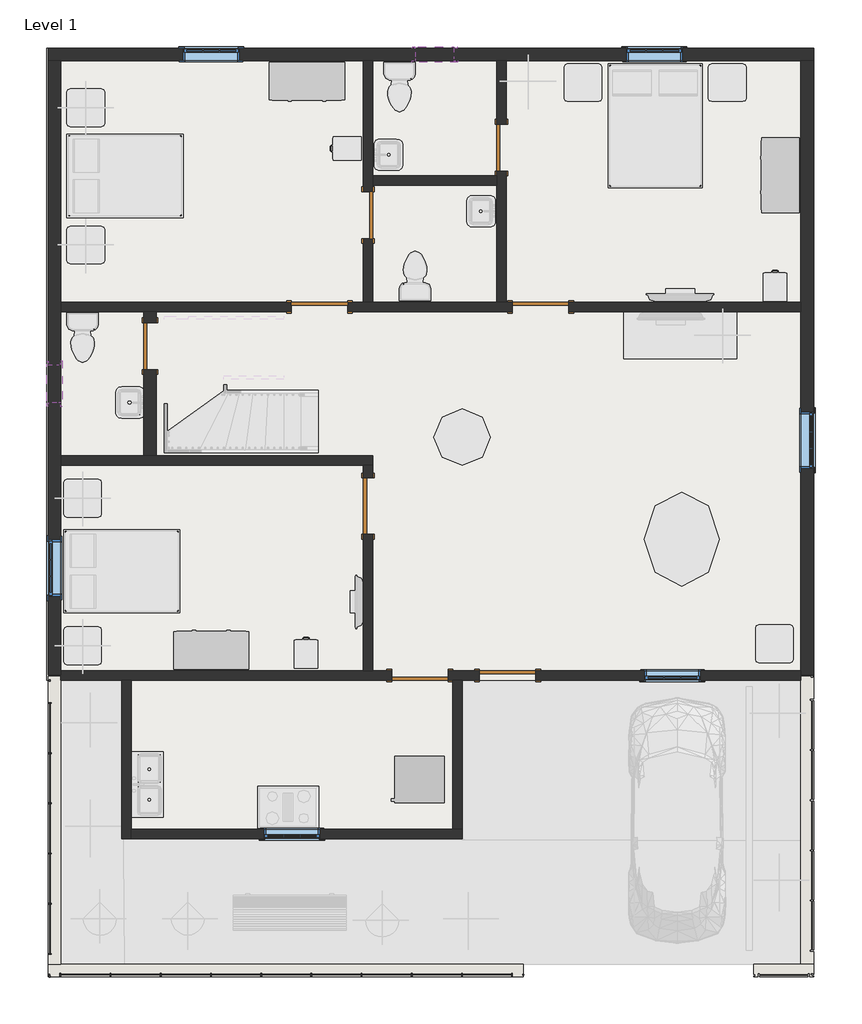
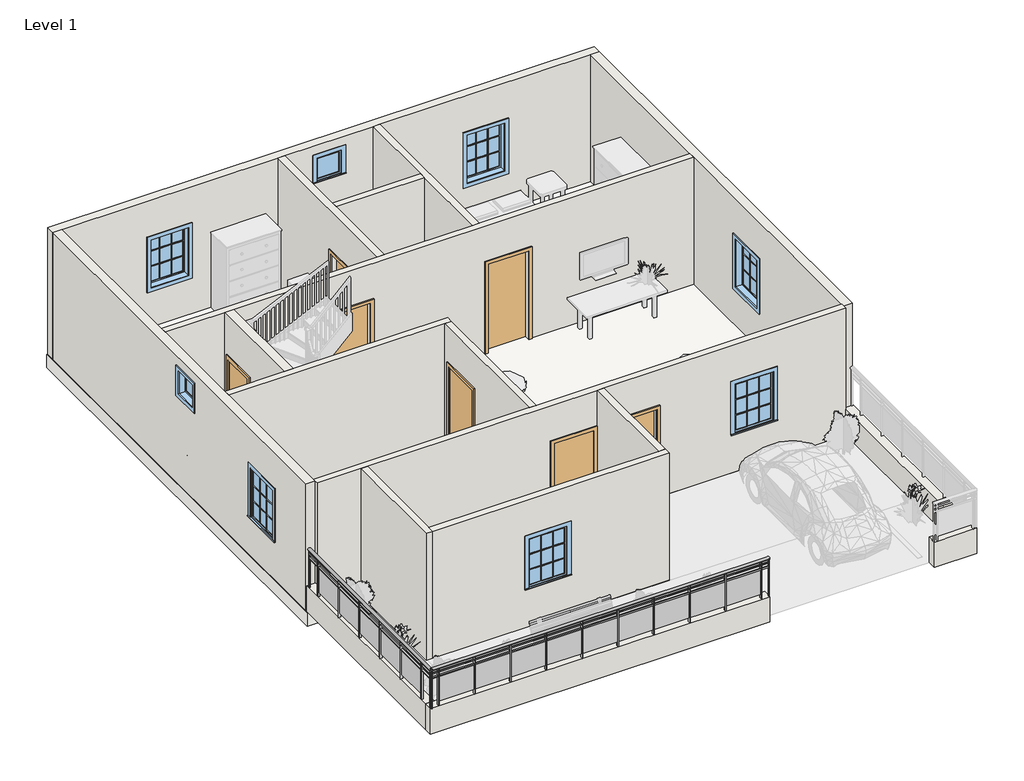
# One storey, part 1 of 3: 18 walls, 8 doors, 8 windows, 2 railings, 1 slab.
"""IFC4 building model written with IfcOpenShell, lengths in millimetres."""

from ifc_helpers import new_model, si_unit, point, frame, origin, origin_with_axes, place, context, project, spatial, polyline, ellipse_curve, trimmed, outline, extrude, faceted_brep, transform, mapped, element, save
from ifc_brep_helpers import plane_surface, extruded_surface, advanced_brep
from components import door_255cab33, door_53b1b562, door_16372e1c, door_686f89d2, window_29c06734, window_5c190c7e, window_e41d21a6

model = new_model("IFC4")

# Units and contexts
model_context = context("Model", 3, world=origin())
ifc_project = project(units=[si_unit("LENGTHUNIT", "METRE", prefix="MILLI")], contexts=[model_context])

# Site, building, storey
site = spatial("IfcSite", under=ifc_project)
building = spatial("IfcBuilding", under=site)
storey = spatial("IfcBuildingStorey", under=building, Name="Level 1", Elevation=0.0)

# Doors
placement = place(None, origin())
door_shape = door_255cab33(model_context)
element("IfcDoor", 1, ObjectType="Single-Flush : 30\" x 80\"", at=placement, inside=storey, context=model_context, shape_type="MappedRepresentation", body=[
    mapped(door_shape, transform((-8429.0402453, 9450.3116886, 0.0), x_axis=(0.0, 1.0, 0.0), y_axis=(-1.0, 0.0, 0.0), z_axis=(0.0, 0.0, 1.0))),
])
element("IfcDoor", 2, ObjectType="Single-Flush : 30\" x 80\"", at=placement, inside=storey, context=model_context, shape_type="MappedRepresentation", body=[
    mapped(door_shape, transform((-6270.0402453, 10542.5116886, 0.0), x_axis=(0.0, -1.0, 0.0), y_axis=(1.0, 0.0, 0.0), z_axis=(0.0, 0.0, 1.0))),
])
door_2_shape = door_53b1b562(model_context)
element("IfcDoor", 3, ObjectType="Single-Flush : 30\" x 80\"", at=placement, inside=storey, context=model_context, shape_type="MappedRepresentation", body=[
    mapped(door_2_shape, transform((-11959.6402453, 7329.4116886, 0.0), x_axis=(0.0, -1.0, 0.0), y_axis=(1.0, 0.0, 0.0), z_axis=(0.0, 0.0, 1.0))),
])
door_3_shape = door_16372e1c(model_context)
element("IfcDoor", 4, ObjectType="Single-Flush : 36\" x 84\"", at=placement, inside=storey, context=model_context, shape_type="MappedRepresentation", body=[
    mapped(door_3_shape, transform((-9216.4402453, 7964.4116886, 0.0), x_axis=(1.0, 0.0, 0.0), y_axis=(0.0, 1.0, 0.0), z_axis=(0.0, 0.0, 1.0))),
])
element("IfcDoor", 5, ObjectType="Single-Flush : 36\" x 84\"", at=placement, inside=storey, context=model_context, shape_type="MappedRepresentation", body=[
    mapped(door_3_shape, transform((-8429.0402453, 4738.6116886, 0.0), x_axis=(0.0, 1.0, 0.0), y_axis=(-1.0, 0.0, 0.0), z_axis=(0.0, 0.0, 1.0))),
])
element("IfcDoor", 6, ObjectType="Single-Flush : 36\" x 84\"", at=placement, inside=storey, context=model_context, shape_type="MappedRepresentation", body=[
    mapped(door_3_shape, transform((-6168.4402453, 1995.4116886, 0.0), x_axis=(1.0, 0.0, 0.0), y_axis=(0.0, 1.0, 0.0), z_axis=(0.0, 0.0, 1.0))),
])
door_4_shape = door_686f89d2(model_context)
element("IfcDoor", 7, ObjectType="Single-Flush : 36\" x 84\"", at=placement, inside=storey, context=model_context, shape_type="MappedRepresentation", body=[
    mapped(door_4_shape, transform((-5635.0402453, 7964.4116886, 0.0), x_axis=(-1.0, 0.0, 0.0), y_axis=(0.0, -1.0, 0.0), z_axis=(0.0, 0.0, 1.0))),
])
element("IfcDoor", 8, ObjectType="Single-Flush : 36\" x 84\"", at=placement, inside=storey, context=model_context, shape_type="MappedRepresentation", body=[
    mapped(door_4_shape, transform((-7590.8402453, 1995.4116886, 0.0), x_axis=(1.0, 0.0, 0.0), y_axis=(0.0, 1.0, 0.0), z_axis=(0.0, 0.0, 1.0))),
])

# Railings
element("IfcRailing", 9, ObjectType="Glass Panel - Bottom Fill", at=placement, inside=storey, context=model_context, shape_type="SolidModel", body=[
    advanced_brep(
    [(-13547.1402453, 1919.2116886, 1524.0), (-13623.3402453, 1919.2116886, 1524.0), (-13547.1402453, -2881.3883114, 1524.0), (-13623.3402453, -2881.3883114, 1524.0)],
    [
        (0, 1, ellipse_curve(frame((-13585.2402453, 1919.2116886, 1524.0), z_axis=(0.0, 1.0, 0.0), x_axis=(-1.0, 0.0, 0.0)), 38.1, 28.575)),
        (1, 0, ellipse_curve(frame((-13585.2402453, 1919.2116886, 1524.0), z_axis=(0.0, 1.0, 0.0), x_axis=(-1.0, 0.0, 0.0)), 38.1, 28.575)),
        (2, 3, ellipse_curve(frame((-13585.2402453, -2881.3883114, 1524.0), z_axis=(0.0, -1.0, 0.0), x_axis=(-1.0, 0.0, 0.0)), 38.1, 28.575)),
        (3, 2, ellipse_curve(frame((-13585.2402453, -2881.3883114, 1524.0), z_axis=(0.0, -1.0, 0.0), x_axis=(-1.0, 0.0, 0.0)), 38.1, 28.575)),
        (0, 2),
        (3, 1),
    ],
    [
        plane_surface(frame((-13585.2402453, 1919.2116886, 1524.0), z_axis=(0.0, 1.0, 0.0), x_axis=(0.0, 0.0, -1.0))),
        plane_surface(frame((-13585.2402453, -2881.3883114, 1524.0), z_axis=(0.0, -1.0, 0.0), x_axis=(0.0, 0.0, -1.0))),
        extruded_surface(trimmed(ellipse_curve(frame((-13585.2402453, -2881.3883114, 1524.0), z_axis=(0.0, 1.0, 0.0), x_axis=(-1.0, 0.0, 0.0)), 38.1, 28.575), [point((-13547.1402453, -2881.3883114, 1524.0))], [point((-13623.3402453, -2881.3883114, 1524.0))], True, "CARTESIAN"), (0.0, 4800.6, 0.0), 4800.6),
        extruded_surface(trimmed(ellipse_curve(frame((-13585.2402453, -2881.3883114, 1524.0), z_axis=(0.0, 1.0, 0.0), x_axis=(-1.0, 0.0, 0.0)), 38.1, 28.575), [point((-13623.3402453, -2881.3883114, 1524.0))], [point((-13547.1402453, -2881.3883114, 1524.0))], True, "CARTESIAN"), (0.0, 4800.6, 0.0), 4800.6),
    ],
    [
        (0, [[1, 2]]),
        (1, [[3, 4]]),
        (2, [[-1, 5, -4, 6]]),
        (3, [[-2, -6, -3, -5]]),
    ],
),
    extrude(outline(polyline([(-13597.9402453, 1919.2116886), (-13572.5402453, 1919.2116886), (-13572.5402453, -2881.3883114), (-13597.9402453, -2881.3883114), (-13597.9402453, 1919.2116886)])), frame((0.0, 0.0, 1409.7), z_axis=(0.0, 0.0, 1.0), x_axis=(1.0, 0.0, 0.0)), (0.0, 0.0, 1.0), 25.4),
    extrude(outline(polyline([(-13597.9402453, 1919.2116886), (-13572.5402453, 1919.2116886), (-13572.5402453, -2881.3883114), (-13597.9402453, -2881.3883114), (-13597.9402453, 1919.2116886)])), frame((0.0, 0.0, 1308.1), z_axis=(0.0, 0.0, 1.0), x_axis=(1.0, 0.0, 0.0)), (0.0, 0.0, 1.0), 25.4),
    extrude(outline(polyline([(-13610.6402453, -2506.7383114), (-13559.8402453, -2506.7383114), (-13559.8402453, -2519.4383114), (-13610.6402453, -2519.4383114), (-13610.6402453, -2506.7383114)])), frame((0.0, 0.0, 609.6), z_axis=(0.0, 0.0, 1.0), x_axis=(1.0, 0.0, 0.0)), (0.0, 0.0, 1.0), 885.6788223),
    extrude(outline(polyline([(-13578.7050883, -1700.2883114), (-13578.7050883, -2513.0883114), (-13585.0550883, -2513.0883114), (-13585.0550883, -1700.2883114), (-13578.7050883, -1700.2883114)])), frame((0.0, 0.0, 711.2), z_axis=(0.0, 0.0, 1.0), x_axis=(1.0, 0.0, 0.0)), (0.0, 0.0, 1.0), 596.9),
    extrude(outline(polyline([(-13610.6402453, -1693.9383114), (-13559.8402453, -1693.9383114), (-13559.8402453, -1706.6383114), (-13610.6402453, -1706.6383114), (-13610.6402453, -1693.9383114)])), frame((0.0, 0.0, 609.6), z_axis=(0.0, 0.0, 1.0), x_axis=(1.0, 0.0, 0.0)), (0.0, 0.0, 1.0), 885.6788223),
    extrude(outline(polyline([(-13578.7050883, -887.4883114), (-13578.7050883, -1700.2883114), (-13585.0550883, -1700.2883114), (-13585.0550883, -887.4883114), (-13578.7050883, -887.4883114)])), frame((0.0, 0.0, 711.2), z_axis=(0.0, 0.0, 1.0), x_axis=(1.0, 0.0, 0.0)), (0.0, 0.0, 1.0), 596.9),
    extrude(outline(polyline([(-13610.6402453, -881.1383114), (-13559.8402453, -881.1383114), (-13559.8402453, -893.8383114), (-13610.6402453, -893.8383114), (-13610.6402453, -881.1383114)])), frame((0.0, 0.0, 609.6), z_axis=(0.0, 0.0, 1.0), x_axis=(1.0, 0.0, 0.0)), (0.0, 0.0, 1.0), 885.6788223),
    extrude(outline(polyline([(-13578.7050883, -74.6883114), (-13578.7050883, -887.4883114), (-13585.0550883, -887.4883114), (-13585.0550883, -74.6883114), (-13578.7050883, -74.6883114)])), frame((0.0, 0.0, 711.2), z_axis=(0.0, 0.0, 1.0), x_axis=(1.0, 0.0, 0.0)), (0.0, 0.0, 1.0), 596.9),
    extrude(outline(polyline([(-13610.6402453, -68.3383114), (-13559.8402453, -68.3383114), (-13559.8402453, -81.0383114), (-13610.6402453, -81.0383114), (-13610.6402453, -68.3383114)])), frame((0.0, 0.0, 609.6), z_axis=(0.0, 0.0, 1.0), x_axis=(1.0, 0.0, 0.0)), (0.0, 0.0, 1.0), 885.6788223),
    extrude(outline(polyline([(-13578.7050883, 738.1116886), (-13578.7050883, -74.6883114), (-13585.0550883, -74.6883114), (-13585.0550883, 738.1116886), (-13578.7050883, 738.1116886)])), frame((0.0, 0.0, 711.2), z_axis=(0.0, 0.0, 1.0), x_axis=(1.0, 0.0, 0.0)), (0.0, 0.0, 1.0), 596.9),
    extrude(outline(polyline([(-13610.6402453, 744.4616886), (-13559.8402453, 744.4616886), (-13559.8402453, 731.7616886), (-13610.6402453, 731.7616886), (-13610.6402453, 744.4616886)])), frame((0.0, 0.0, 609.6), z_axis=(0.0, 0.0, 1.0), x_axis=(1.0, 0.0, 0.0)), (0.0, 0.0, 1.0), 885.6788223),
    extrude(outline(polyline([(-13578.7050883, 1550.9116886), (-13578.7050883, 738.1116886), (-13585.0550883, 738.1116886), (-13585.0550883, 1550.9116886), (-13578.7050883, 1550.9116886)])), frame((0.0, 0.0, 711.2), z_axis=(0.0, 0.0, 1.0), x_axis=(1.0, 0.0, 0.0)), (0.0, 0.0, 1.0), 596.9),
    extrude(outline(polyline([(-13610.6402453, 1557.2616886), (-13559.8402453, 1557.2616886), (-13559.8402453, 1544.5616886), (-13610.6402453, 1544.5616886), (-13610.6402453, 1557.2616886)])), frame((0.0, 0.0, 609.6), z_axis=(0.0, 0.0, 1.0), x_axis=(1.0, 0.0, 0.0)), (0.0, 0.0, 1.0), 885.6788223),
    extrude(outline(polyline([(-13594.7652453, -2868.6883114), (-13575.7152453, -2868.6883114), (-13575.7152453, -2887.7383114), (-13594.7652453, -2887.7383114), (-13594.7652453, -2868.6883114)])), frame((0.0, 0.0, 609.6), z_axis=(0.0, 0.0, 1.0), x_axis=(1.0, 0.0, 0.0)), (0.0, 0.0, 1.0), 885.6788223),
    extrude(outline(polyline([(-13594.7652453, 1925.5616886), (-13575.7152453, 1925.5616886), (-13575.7152453, 1906.5116886), (-13594.7652453, 1906.5116886), (-13594.7652453, 1925.5616886)])), frame((0.0, 0.0, 609.6), z_axis=(0.0, 0.0, 1.0), x_axis=(1.0, 0.0, 0.0)), (0.0, 0.0, 1.0), 885.6788223),
])
element("IfcRailing", 10, ObjectType="Glass Panel - Bottom Fill", at=placement, inside=storey, context=model_context, shape_type="SolidModel", body=[
    advanced_brep(
    [(-13594.7652453, -2814.7133114, 1524.0), (-13594.7652453, -2890.9133114, 1524.0), (-5914.4402453, -2814.7133114, 1524.0), (-5914.4402453, -2890.9133114, 1524.0)],
    [
        (0, 1, ellipse_curve(frame((-13594.7652453, -2852.8133114, 1524.0), z_axis=(-1.0, 0.0, 0.0), x_axis=(0.0, -1.0, 0.0)), 38.1, 28.575)),
        (1, 0, ellipse_curve(frame((-13594.7652453, -2852.8133114, 1524.0), z_axis=(-1.0, 0.0, 0.0), x_axis=(0.0, -1.0, 0.0)), 38.1, 28.575)),
        (2, 3, ellipse_curve(frame((-5914.4402453, -2852.8133114, 1524.0), z_axis=(1.0, 0.0, 0.0), x_axis=(0.0, -1.0, 0.0)), 38.1, 28.575)),
        (3, 2, ellipse_curve(frame((-5914.4402453, -2852.8133114, 1524.0), z_axis=(1.0, 0.0, 0.0), x_axis=(0.0, -1.0, 0.0)), 38.1, 28.575)),
        (0, 2),
        (3, 1),
    ],
    [
        plane_surface(frame((-13594.7652453, -2852.8133114, 1524.0), z_axis=(-1.0, 0.0, 0.0), x_axis=(0.0, 1.0, 0.0))),
        plane_surface(frame((-5914.4402453, -2852.8133114, 1524.0), z_axis=(1.0, 0.0, 0.0), x_axis=(0.0, 1.0, 0.0))),
        extruded_surface(trimmed(ellipse_curve(frame((-5914.4402453, -2852.8133114, 1524.0), z_axis=(-1.0, 0.0, 0.0), x_axis=(0.0, -1.0, 0.0)), 38.1, 28.575), [point((-5914.4402453, -2814.7133114, 1524.0))], [point((-5914.4402453, -2890.9133114, 1524.0))], True, "CARTESIAN"), (-7680.324999999999, 0.0, 0.0), 7680.324999999999),
        extruded_surface(trimmed(ellipse_curve(frame((-5914.4402453, -2852.8133114, 1524.0), z_axis=(-1.0, 0.0, 0.0), x_axis=(0.0, -1.0, 0.0)), 38.1, 28.575), [point((-5914.4402453, -2890.9133114, 1524.0))], [point((-5914.4402453, -2814.7133114, 1524.0))], True, "CARTESIAN"), (-7680.324999999999, 0.0, 0.0), 7680.324999999999),
    ],
    [
        (0, [[1, 2]]),
        (1, [[3, 4]]),
        (2, [[-1, 5, -4, 6]]),
        (3, [[-2, -6, -3, -5]]),
    ],
),
    extrude(outline(polyline([(-13594.7652453, -2865.5133114), (-13594.7652453, -2840.1133114), (-5914.4402453, -2840.1133114), (-5914.4402453, -2865.5133114), (-13594.7652453, -2865.5133114)])), frame((0.0, 0.0, 1409.7), z_axis=(0.0, 0.0, 1.0), x_axis=(1.0, 0.0, 0.0)), (0.0, 0.0, 1.0), 25.4),
    extrude(outline(polyline([(-13594.7652453, -2865.5133114), (-13594.7652453, -2840.1133114), (-5914.4402453, -2840.1133114), (-5914.4402453, -2865.5133114), (-13594.7652453, -2865.5133114)])), frame((0.0, 0.0, 1308.1), z_axis=(0.0, 0.0, 1.0), x_axis=(1.0, 0.0, 0.0)), (0.0, 0.0, 1.0), 25.4),
    extrude(outline(polyline([(-6103.3527453, -2878.2133114), (-6103.3527453, -2827.4133114), (-6090.6527453, -2827.4133114), (-6090.6527453, -2878.2133114), (-6103.3527453, -2878.2133114)])), frame((0.0, 0.0, 609.6), z_axis=(0.0, 0.0, 1.0), x_axis=(1.0, 0.0, 0.0)), (0.0, 0.0, 1.0), 885.6788223),
    extrude(outline(polyline([(-6909.8027453, -2846.2781544), (-6097.0027453, -2846.2781544), (-6097.0027453, -2852.6281544), (-6909.8027453, -2852.6281544), (-6909.8027453, -2846.2781544)])), frame((0.0, 0.0, 711.2), z_axis=(0.0, 0.0, 1.0), x_axis=(1.0, 0.0, 0.0)), (0.0, 0.0, 1.0), 596.9),
    extrude(outline(polyline([(-6916.1527453, -2878.2133114), (-6916.1527453, -2827.4133114), (-6903.4527453, -2827.4133114), (-6903.4527453, -2878.2133114), (-6916.1527453, -2878.2133114)])), frame((0.0, 0.0, 609.6), z_axis=(0.0, 0.0, 1.0), x_axis=(1.0, 0.0, 0.0)), (0.0, 0.0, 1.0), 885.6788223),
    extrude(outline(polyline([(-7722.6027453, -2846.2781544), (-6909.8027453, -2846.2781544), (-6909.8027453, -2852.6281544), (-7722.6027453, -2852.6281544), (-7722.6027453, -2846.2781544)])), frame((0.0, 0.0, 711.2), z_axis=(0.0, 0.0, 1.0), x_axis=(1.0, 0.0, 0.0)), (0.0, 0.0, 1.0), 596.9),
    extrude(outline(polyline([(-7728.9527453, -2878.2133114), (-7728.9527453, -2827.4133114), (-7716.2527453, -2827.4133114), (-7716.2527453, -2878.2133114), (-7728.9527453, -2878.2133114)])), frame((0.0, 0.0, 609.6), z_axis=(0.0, 0.0, 1.0), x_axis=(1.0, 0.0, 0.0)), (0.0, 0.0, 1.0), 885.6788223),
    extrude(outline(polyline([(-8535.4027453, -2846.2781544), (-7722.6027453, -2846.2781544), (-7722.6027453, -2852.6281544), (-8535.4027453, -2852.6281544), (-8535.4027453, -2846.2781544)])), frame((0.0, 0.0, 711.2), z_axis=(0.0, 0.0, 1.0), x_axis=(1.0, 0.0, 0.0)), (0.0, 0.0, 1.0), 596.9),
    extrude(outline(polyline([(-8541.7527453, -2878.2133114), (-8541.7527453, -2827.4133114), (-8529.0527453, -2827.4133114), (-8529.0527453, -2878.2133114), (-8541.7527453, -2878.2133114)])), frame((0.0, 0.0, 609.6), z_axis=(0.0, 0.0, 1.0), x_axis=(1.0, 0.0, 0.0)), (0.0, 0.0, 1.0), 885.6788223),
    extrude(outline(polyline([(-9348.2027453, -2846.2781544), (-8535.4027453, -2846.2781544), (-8535.4027453, -2852.6281544), (-9348.2027453, -2852.6281544), (-9348.2027453, -2846.2781544)])), frame((0.0, 0.0, 711.2), z_axis=(0.0, 0.0, 1.0), x_axis=(1.0, 0.0, 0.0)), (0.0, 0.0, 1.0), 596.9),
    extrude(outline(polyline([(-9354.5527453, -2878.2133114), (-9354.5527453, -2827.4133114), (-9341.8527453, -2827.4133114), (-9341.8527453, -2878.2133114), (-9354.5527453, -2878.2133114)])), frame((0.0, 0.0, 609.6), z_axis=(0.0, 0.0, 1.0), x_axis=(1.0, 0.0, 0.0)), (0.0, 0.0, 1.0), 885.6788223),
    extrude(outline(polyline([(-10161.0027453, -2846.2781544), (-9348.2027453, -2846.2781544), (-9348.2027453, -2852.6281544), (-10161.0027453, -2852.6281544), (-10161.0027453, -2846.2781544)])), frame((0.0, 0.0, 711.2), z_axis=(0.0, 0.0, 1.0), x_axis=(1.0, 0.0, 0.0)), (0.0, 0.0, 1.0), 596.9),
    extrude(outline(polyline([(-10167.3527453, -2878.2133114), (-10167.3527453, -2827.4133114), (-10154.6527453, -2827.4133114), (-10154.6527453, -2878.2133114), (-10167.3527453, -2878.2133114)])), frame((0.0, 0.0, 609.6), z_axis=(0.0, 0.0, 1.0), x_axis=(1.0, 0.0, 0.0)), (0.0, 0.0, 1.0), 885.6788223),
    extrude(outline(polyline([(-10973.8027453, -2846.2781544), (-10161.0027453, -2846.2781544), (-10161.0027453, -2852.6281544), (-10973.8027453, -2852.6281544), (-10973.8027453, -2846.2781544)])), frame((0.0, 0.0, 711.2), z_axis=(0.0, 0.0, 1.0), x_axis=(1.0, 0.0, 0.0)), (0.0, 0.0, 1.0), 596.9),
    extrude(outline(polyline([(-10980.1527453, -2878.2133114), (-10980.1527453, -2827.4133114), (-10967.4527453, -2827.4133114), (-10967.4527453, -2878.2133114), (-10980.1527453, -2878.2133114)])), frame((0.0, 0.0, 609.6), z_axis=(0.0, 0.0, 1.0), x_axis=(1.0, 0.0, 0.0)), (0.0, 0.0, 1.0), 885.6788223),
    extrude(outline(polyline([(-11786.6027453, -2846.2781544), (-10973.8027453, -2846.2781544), (-10973.8027453, -2852.6281544), (-11786.6027453, -2852.6281544), (-11786.6027453, -2846.2781544)])), frame((0.0, 0.0, 711.2), z_axis=(0.0, 0.0, 1.0), x_axis=(1.0, 0.0, 0.0)), (0.0, 0.0, 1.0), 596.9),
    extrude(outline(polyline([(-11792.9527453, -2878.2133114), (-11792.9527453, -2827.4133114), (-11780.2527453, -2827.4133114), (-11780.2527453, -2878.2133114), (-11792.9527453, -2878.2133114)])), frame((0.0, 0.0, 609.6), z_axis=(0.0, 0.0, 1.0), x_axis=(1.0, 0.0, 0.0)), (0.0, 0.0, 1.0), 885.6788223),
    extrude(outline(polyline([(-12599.4027453, -2846.2781544), (-11786.6027453, -2846.2781544), (-11786.6027453, -2852.6281544), (-12599.4027453, -2852.6281544), (-12599.4027453, -2846.2781544)])), frame((0.0, 0.0, 711.2), z_axis=(0.0, 0.0, 1.0), x_axis=(1.0, 0.0, 0.0)), (0.0, 0.0, 1.0), 596.9),
    extrude(outline(polyline([(-12605.7527453, -2878.2133114), (-12605.7527453, -2827.4133114), (-12593.0527453, -2827.4133114), (-12593.0527453, -2878.2133114), (-12605.7527453, -2878.2133114)])), frame((0.0, 0.0, 609.6), z_axis=(0.0, 0.0, 1.0), x_axis=(1.0, 0.0, 0.0)), (0.0, 0.0, 1.0), 885.6788223),
    extrude(outline(polyline([(-13412.2027453, -2846.2781544), (-12599.4027453, -2846.2781544), (-12599.4027453, -2852.6281544), (-13412.2027453, -2852.6281544), (-13412.2027453, -2846.2781544)])), frame((0.0, 0.0, 711.2), z_axis=(0.0, 0.0, 1.0), x_axis=(1.0, 0.0, 0.0)), (0.0, 0.0, 1.0), 596.9),
    extrude(outline(polyline([(-13418.5527453, -2878.2133114), (-13418.5527453, -2827.4133114), (-13405.8527453, -2827.4133114), (-13405.8527453, -2878.2133114), (-13418.5527453, -2878.2133114)])), frame((0.0, 0.0, 609.6), z_axis=(0.0, 0.0, 1.0), x_axis=(1.0, 0.0, 0.0)), (0.0, 0.0, 1.0), 885.6788223),
    extrude(outline(polyline([(-5927.1402453, -2862.3383114), (-5927.1402453, -2843.2883114), (-5908.0902453, -2843.2883114), (-5908.0902453, -2862.3383114), (-5927.1402453, -2862.3383114)])), frame((0.0, 0.0, 609.6), z_axis=(0.0, 0.0, 1.0), x_axis=(1.0, 0.0, 0.0)), (0.0, 0.0, 1.0), 885.6788223),
    extrude(outline(polyline([(-13601.1152453, -2862.3383114), (-13601.1152453, -2843.2883114), (-13582.0652453, -2843.2883114), (-13582.0652453, -2862.3383114), (-13601.1152453, -2862.3383114)])), frame((0.0, 0.0, 609.6), z_axis=(0.0, 0.0, 1.0), x_axis=(1.0, 0.0, 0.0)), (0.0, 0.0, 1.0), 885.6788223),
])

# Slab
element("IfcSlab", 11, ObjectType="Generic - 12\"", at=placement, inside=storey, context=model_context, shape_type="SweptSolid", body=[
    extrude(outline(polyline([(-1215.4402453, 12155.4116886), (-1215.4402453, 1919.2116886), (-6905.0402453, 1919.2116886), (-6905.0402453, -646.1883114), (-12416.8402453, -646.1883114), (-12416.8402453, 1919.2116886), (-13636.0402453, 1919.2116886), (-13636.0402453, 12155.4116886), (-1215.4402453, 12155.4116886)])), frame((0.0, 0.0, -304.8), z_axis=(0.0, 0.0, 1.0), x_axis=(1.0, 0.0, 0.0)), (0.0, 0.0, 1.0), 304.8),
])

# Walls
element("IfcWall", 12, ObjectType="Generic - 2", at=placement, inside=storey, context=model_context, shape_type="Brep", body=[
    faceted_brep([(-1215.4402453, -2678.1883114, 0.0), (-1418.6402453, -2678.1883114, 0.0), (-2180.6402453, -2678.1883114, 0.0), (-2180.6402453, -2678.1883114, 609.6), (-1418.6402453, -2678.1883114, 609.6), (-1215.4402453, -2678.1883114, 609.6), (-1215.4402453, -2881.3883114, 0.0), (-1215.4402453, -2881.3883114, 609.6), (-2180.6402453, -2881.3883114, 609.6), (-2180.6402453, -2881.3883114, 0.0)], [[[0, 1, 2, 3, 4, 5]], [[6, 7, 8, 9]], [[2, 1, 0, 6, 9]], [[3, 2, 9, 8]], [[5, 4, 3, 8, 7]], [[0, 5, 7, 6]]]),
])
element("IfcWall", 13, ObjectType="Generic - 2", at=placement, inside=storey, context=model_context, shape_type="SweptSolid", body=[
    extrude(outline(polyline([(-13407.4402453, 1982.7116886), (-13407.4402453, -2678.1883114), (-13610.6402453, -2678.1883114), (-13610.6402453, 1982.7116886), (-13407.4402453, 1982.7116886)])), origin_with_axes(), (0.0, 0.0, 1.0), 609.6),
])
element("IfcWall", 14, ObjectType="Generic - 2", at=placement, inside=storey, context=model_context, shape_type="Brep", body=[
    faceted_brep([(-1418.6402453, 1982.7116886, 0.0), (-1418.6402453, 1919.2116886, 0.0), (-1418.6402453, -2678.1883114, 0.0), (-1418.6402453, -2678.1883114, 609.6), (-1418.6402453, 1982.7116886, 609.6), (-1215.4402453, 1982.7116886, 0.0), (-1215.4402453, 1982.7116886, 609.6), (-1215.4402453, -2678.1883114, 609.6), (-1215.4402453, -2678.1883114, 0.0)], [[[0, 1, 2, 3, 4]], [[5, 6, 7, 8]], [[2, 1, 0, 5, 8]], [[4, 3, 7, 6]], [[0, 4, 6, 5]], [[3, 2, 8, 7]]]),
])
element("IfcWall", 15, ObjectType="Generic - 2", at=placement, inside=storey, context=model_context, shape_type="Brep", body=[
    faceted_brep([(-5914.4402453, -2678.1883114, 0.0), (-13407.4402453, -2678.1883114, 0.0), (-13610.6402453, -2678.1883114, 0.0), (-13610.6402453, -2678.1883114, 609.6), (-13407.4402453, -2678.1883114, 609.6), (-5914.4402453, -2678.1883114, 609.6), (-5914.4402453, -2881.3883114, 0.0), (-5914.4402453, -2881.3883114, 609.6), (-13610.6402453, -2881.3883114, 609.6), (-13610.6402453, -2881.3883114, 0.0)], [[[0, 1, 2, 3, 4, 5]], [[6, 7, 8, 9]], [[2, 1, 0, 6, 9]], [[5, 4, 3, 8, 7]], [[0, 5, 7, 6]], [[3, 2, 9, 8]]]),
])
element("IfcWall", 16, ObjectType="Generic - 8\"", at=placement, inside=storey, context=model_context, shape_type="Brep", body=[
    faceted_brep([(-13610.6402453, 11952.2116886, 0.0), (-13407.4402453, 11952.2116886, 0.0), (-8505.2402453, 11952.2116886, 0.0), (-8352.8402453, 11952.2116886, 0.0), (-6346.2402453, 11952.2116886, 0.0), (-6193.8402453, 11952.2116886, 0.0), (-1418.6402453, 11952.2116886, 0.0), (-1215.4402453, 11952.2116886, 0.0), (-1215.4402453, 11952.2116886, 3048.0), (-1418.6402453, 11952.2116886, 3048.0), (-6193.8402453, 11952.2116886, 3048.0), (-6346.2402453, 11952.2116886, 3048.0), (-8352.8402453, 11952.2116886, 3048.0), (-8505.2402453, 11952.2116886, 3048.0), (-13407.4402453, 11952.2116886, 3048.0), (-13610.6402453, 11952.2116886, 3048.0), (-10511.8402453, 11952.2116886, 2133.6), (-10511.8402453, 11952.2116886, 914.4), (-11426.2402453, 11952.2116886, 914.4), (-11426.2402453, 11952.2116886, 2133.6), (-3336.3402453, 11952.2116886, 2133.6), (-3336.3402453, 11952.2116886, 914.4), (-4250.7402453, 11952.2116886, 914.4), (-4250.7402453, 11952.2116886, 2133.6), (-7654.3402453, 11952.2116886, 2768.6), (-7044.7402453, 11952.2116886, 2768.6), (-7044.7402453, 11952.2116886, 2159.0), (-7654.3402453, 11952.2116886, 2159.0), (-13610.6402453, 12155.4116886, 0.0), (-13610.6402453, 12155.4116886, 3048.0), (-1215.4402453, 12155.4116886, 3048.0), (-1215.4402453, 12155.4116886, 0.0), (-10511.8402453, 12155.4116886, 2133.6), (-11426.2402453, 12155.4116886, 2133.6), (-11426.2402453, 12155.4116886, 914.4), (-10511.8402453, 12155.4116886, 914.4), (-3336.3402453, 12155.4116886, 2133.6), (-4250.7402453, 12155.4116886, 2133.6), (-4250.7402453, 12155.4116886, 914.4), (-3336.3402453, 12155.4116886, 914.4), (-7654.3402453, 12155.4116886, 2768.6), (-7654.3402453, 12155.4116886, 2159.0), (-7044.7402453, 12155.4116886, 2159.0), (-7044.7402453, 12155.4116886, 2768.6)], [[[0, 1, 2, 3, 4, 5, 6, 7, 8, 9, 10, 11, 12, 13, 14, 15], [16, 17, 18, 19], [20, 21, 22, 23], [24, 25, 26, 27]], [[28, 29, 30, 31], [32, 33, 34, 35], [36, 37, 38, 39], [40, 41, 42, 43]], [[7, 6, 5, 4, 3, 2, 1, 0, 28, 31]], [[8, 7, 31, 30]], [[0, 15, 29, 28]], [[17, 16, 32, 35]], [[18, 17, 35, 34]], [[19, 18, 34, 33]], [[16, 19, 33, 32]], [[21, 20, 36, 39]], [[22, 21, 39, 38]], [[23, 22, 38, 37]], [[20, 23, 37, 36]], [[41, 40, 24, 27]], [[42, 41, 27, 26]], [[43, 42, 26, 25]], [[40, 43, 25, 24]], [[15, 14, 13, 12, 11, 10, 9, 8, 30, 29]]]),
])
element("IfcWall", 17, ObjectType="Generic - 8\"", at=placement, inside=storey, context=model_context, shape_type="Brep", body=[
    faceted_brep([(-1418.6402453, 11952.2116886, 0.0), (-1418.6402453, 8040.6116886, 0.0), (-1418.6402453, 7888.2116886, 0.0), (-1418.6402453, 2008.1116886, 0.0), (-1418.6402453, 2008.1116886, 3048.0), (-1418.6402453, 7888.2116886, 3048.0), (-1418.6402453, 8040.6116886, 3048.0), (-1418.6402453, 11952.2116886, 3048.0), (-1418.6402453, 5348.2116886, 2133.6), (-1418.6402453, 5348.2116886, 914.4), (-1418.6402453, 6262.6116886, 914.4), (-1418.6402453, 6262.6116886, 2133.6), (-1215.4402453, 11952.2116886, 0.0), (-1215.4402453, 11952.2116886, 3048.0), (-1215.4402453, 2008.1116886, 3048.0), (-1215.4402453, 2008.1116886, 0.0), (-1215.4402453, 5348.2116886, 2133.6), (-1215.4402453, 6262.6116886, 2133.6), (-1215.4402453, 6262.6116886, 914.4), (-1215.4402453, 5348.2116886, 914.4)], [[[0, 1, 2, 3, 4, 5, 6, 7], [8, 9, 10, 11]], [[12, 13, 14, 15], [16, 17, 18, 19]], [[3, 2, 1, 0, 12, 15]], [[4, 3, 15, 14]], [[0, 7, 13, 12]], [[9, 8, 16, 19]], [[10, 9, 19, 18]], [[11, 10, 18, 17]], [[8, 11, 17, 16]], [[7, 6, 5, 4, 14, 13]]]),
])
element("IfcWall", 18, ObjectType="Generic - 8\"", at=placement, inside=storey, context=model_context, shape_type="SweptSolid", body=[
    extrude(outline(polyline([(6948.4116886, 2032.0), (6948.4116886, 0.0), (5551.4116886, 0.0), (5551.4116886, 3048.0), (7888.2116886, 3048.0), (7888.2116886, 0.0), (7710.4116886, 0.0), (7710.4116886, 2032.0), (6948.4116886, 2032.0)])), frame((-12061.2402453, 0.0, 0.0), z_axis=(1.0, 0.0, 0.0), x_axis=(0.0, 1.0, 0.0)), (0.0, 0.0, 1.0), 203.2),
])
element("IfcWall", 19, ObjectType="Generic - 8\"", at=placement, inside=storey, context=model_context, shape_type="Brep", body=[
    faceted_brep([(-13407.4402453, 2008.1116886, 0.0), (-13407.4402453, 2071.6116886, 0.0), (-13407.4402453, 5399.0116886, 0.0), (-13407.4402453, 5551.4116886, 0.0), (-13407.4402453, 7888.2116886, 0.0), (-13407.4402453, 8040.6116886, 0.0), (-13407.4402453, 11952.2116886, 0.0), (-13407.4402453, 11952.2116886, 3048.0), (-13407.4402453, 8040.6116886, 3048.0), (-13407.4402453, 7888.2116886, 3048.0), (-13407.4402453, 5551.4116886, 3048.0), (-13407.4402453, 5399.0116886, 3048.0), (-13407.4402453, 2071.6116886, 3048.0), (-13407.4402453, 2008.1116886, 3048.0), (-13407.4402453, 4192.5116886, 2133.6), (-13407.4402453, 4192.5116886, 914.4), (-13407.4402453, 3278.1116886, 914.4), (-13407.4402453, 3278.1116886, 2133.6), (-13407.4402453, 6415.0116886, 2768.6), (-13407.4402453, 7024.6116886, 2768.6), (-13407.4402453, 7024.6116886, 2159.0), (-13407.4402453, 6415.0116886, 2159.0), (-13610.6402453, 2008.1116886, 0.0), (-13610.6402453, 2008.1116886, 3048.0), (-13610.6402453, 11952.2116886, 3048.0), (-13610.6402453, 11952.2116886, 0.0), (-13610.6402453, 4192.5116886, 2133.6), (-13610.6402453, 3278.1116886, 2133.6), (-13610.6402453, 3278.1116886, 914.4), (-13610.6402453, 4192.5116886, 914.4), (-13610.6402453, 6415.0116886, 2768.6), (-13610.6402453, 6415.0116886, 2159.0), (-13610.6402453, 7024.6116886, 2159.0), (-13610.6402453, 7024.6116886, 2768.6)], [[[0, 1, 2, 3, 4, 5, 6, 7, 8, 9, 10, 11, 12, 13], [14, 15, 16, 17], [18, 19, 20, 21]], [[22, 23, 24, 25], [26, 27, 28, 29], [30, 31, 32, 33]], [[6, 5, 4, 3, 2, 1, 0, 22, 25]], [[0, 13, 23, 22]], [[7, 6, 25, 24]], [[14, 17, 27, 26]], [[17, 16, 28, 27]], [[16, 15, 29, 28]], [[15, 14, 26, 29]], [[30, 33, 19, 18]], [[33, 32, 20, 19]], [[32, 31, 21, 20]], [[31, 30, 18, 21]], [[13, 12, 11, 10, 9, 8, 7, 24, 23]]]),
])
element("IfcWall", 20, ObjectType="inner wall 6\"", at=placement, inside=storey, context=model_context, shape_type="Brep", body=[
    faceted_brep([(-8505.2402453, 11952.2116886, 0.0), (-8505.2402453, 9831.3116886, 0.0), (-8505.2402453, 9831.3116886, 2032.0), (-8505.2402453, 9069.3116886, 2032.0), (-8505.2402453, 9069.3116886, 0.0), (-8505.2402453, 8040.6116886, 0.0), (-8505.2402453, 8040.6116886, 3048.0), (-8505.2402453, 11952.2116886, 3048.0), (-8352.8402453, 9831.3116886, 2032.0), (-8352.8402453, 9831.3116886, 0.0), (-8352.8402453, 9932.9116886, 0.0), (-8352.8402453, 10085.3116886, 0.0), (-8352.8402453, 11952.2116886, 0.0), (-8352.8402453, 11952.2116886, 3048.0), (-8352.8402453, 10085.3116886, 3048.0), (-8352.8402453, 9932.9116886, 3048.0), (-8352.8402453, 8040.6116886, 3048.0), (-8352.8402453, 8040.6116886, 0.0), (-8352.8402453, 9069.3116886, 0.0), (-8352.8402453, 9069.3116886, 2032.0)], [[[0, 1, 2, 3, 4, 5, 6, 7]], [[8, 9, 10, 11, 12, 13, 14, 15, 16, 17, 18, 19]], [[18, 17, 5, 4]], [[12, 11, 10, 9, 1, 0]], [[0, 7, 13, 12]], [[6, 5, 17, 16]], [[2, 1, 9, 8]], [[3, 2, 8, 19]], [[4, 3, 19, 18]], [[7, 6, 16, 15, 14, 13]]]),
])
element("IfcWall", 21, ObjectType="inner wall 6\"", at=placement, inside=storey, context=model_context, shape_type="Brep", body=[
    faceted_brep([(-6092.2402453, 8040.6116886, 2133.6), (-6092.2402453, 8040.6116886, 0.0), (-6193.8402453, 8040.6116886, 0.0), (-6346.2402453, 8040.6116886, 0.0), (-8352.8402453, 8040.6116886, 0.0), (-8505.2402453, 8040.6116886, 0.0), (-8759.2402453, 8040.6116886, 0.0), (-8759.2402453, 8040.6116886, 2133.6), (-9673.6402453, 8040.6116886, 2133.6), (-9673.6402453, 8040.6116886, 0.0), (-13407.4402453, 8040.6116886, 0.0), (-13407.4402453, 8040.6116886, 3048.0), (-8505.2402453, 8040.6116886, 3048.0), (-8352.8402453, 8040.6116886, 3048.0), (-6346.2402453, 8040.6116886, 3048.0), (-6193.8402453, 8040.6116886, 3048.0), (-1418.6402453, 8040.6116886, 3048.0), (-1418.6402453, 8040.6116886, 0.0), (-5177.8402453, 8040.6116886, 0.0), (-5177.8402453, 8040.6116886, 2133.6), (-8759.2402453, 7888.2116886, 0.0), (-6092.2402453, 7888.2116886, 0.0), (-6092.2402453, 7888.2116886, 2133.6), (-5177.8402453, 7888.2116886, 2133.6), (-5177.8402453, 7888.2116886, 0.0), (-1418.6402453, 7888.2116886, 0.0), (-1418.6402453, 7888.2116886, 3048.0), (-11858.0402453, 7888.2116886, 3048.0), (-12061.2402453, 7888.2116886, 3048.0), (-13407.4402453, 7888.2116886, 3048.0), (-13407.4402453, 7888.2116886, 0.0), (-12061.2402453, 7888.2116886, 0.0), (-11858.0402453, 7888.2116886, 0.0), (-9673.6402453, 7888.2116886, 0.0), (-9673.6402453, 7888.2116886, 2133.6), (-8759.2402453, 7888.2116886, 2133.6)], [[[0, 1, 2, 3, 4, 5, 6, 7, 8, 9, 10, 11, 12, 13, 14, 15, 16, 17, 18, 19]], [[20, 21, 22, 23, 24, 25, 26, 27, 28, 29, 30, 31, 32, 33, 34, 35]], [[18, 17, 25, 24]], [[6, 5, 4, 3, 2, 1, 21, 20]], [[33, 32, 31, 30, 10, 9]], [[11, 10, 30, 29]], [[17, 16, 26, 25]], [[7, 6, 20, 35]], [[8, 7, 35, 34]], [[9, 8, 34, 33]], [[22, 21, 1, 0]], [[23, 22, 0, 19]], [[24, 23, 19, 18]], [[16, 15, 14, 13, 12, 11, 29, 28, 27, 26]]]),
])
element("IfcWall", 22, ObjectType="inner wall 6\"", at=placement, inside=storey, context=model_context, shape_type="Brep", body=[
    faceted_brep([(-6346.2402453, 10161.5116886, 2032.0), (-6346.2402453, 10161.5116886, 0.0), (-6346.2402453, 10085.3116886, 0.0), (-6346.2402453, 9932.9116886, 0.0), (-6346.2402453, 8040.6116886, 0.0), (-6346.2402453, 8040.6116886, 3048.0), (-6346.2402453, 9932.9116886, 3048.0), (-6346.2402453, 10085.3116886, 3048.0), (-6346.2402453, 11952.2116886, 3048.0), (-6346.2402453, 11952.2116886, 0.0), (-6346.2402453, 10923.5116886, 0.0), (-6346.2402453, 10923.5116886, 2032.0), (-6193.8402453, 8040.6116886, 0.0), (-6193.8402453, 10161.5116886, 0.0), (-6193.8402453, 10161.5116886, 2032.0), (-6193.8402453, 10923.5116886, 2032.0), (-6193.8402453, 10923.5116886, 0.0), (-6193.8402453, 11952.2116886, 0.0), (-6193.8402453, 11952.2116886, 3048.0), (-6193.8402453, 8040.6116886, 3048.0)], [[[0, 1, 2, 3, 4, 5, 6, 7, 8, 9, 10, 11]], [[12, 13, 14, 15, 16, 17, 18, 19]], [[10, 9, 17, 16]], [[4, 3, 2, 1, 13, 12]], [[9, 8, 18, 17]], [[5, 4, 12, 19]], [[14, 13, 1, 0]], [[15, 14, 0, 11]], [[16, 15, 11, 10]], [[8, 7, 6, 5, 19, 18]]]),
])
element("IfcWall", 23, ObjectType="inner wall 6\"", at=placement, inside=storey, context=model_context, shape_type="Brep", body=[
    faceted_brep([(-13407.4402453, 5399.0116886, 0.0), (-8505.2402453, 5399.0116886, 0.0), (-8352.8402453, 5399.0116886, 0.0), (-8352.8402453, 5399.0116886, 3048.0), (-8505.2402453, 5399.0116886, 3048.0), (-13407.4402453, 5399.0116886, 3048.0), (-13407.4402453, 5551.4116886, 0.0), (-13407.4402453, 5551.4116886, 3048.0), (-12061.2402453, 5551.4116886, 3048.0), (-11858.0402453, 5551.4116886, 3048.0), (-8352.8402453, 5551.4116886, 3048.0), (-8352.8402453, 5551.4116886, 0.0), (-11858.0402453, 5551.4116886, 0.0), (-12061.2402453, 5551.4116886, 0.0)], [[[0, 1, 2, 3, 4, 5]], [[6, 7, 8, 9, 10, 11, 12, 13]], [[2, 1, 0, 6, 13, 12, 11]], [[0, 5, 7, 6]], [[3, 2, 11, 10]], [[5, 4, 3, 10, 9, 8, 7]]]),
])
element("IfcWall", 24, ObjectType="inner wall 6\"", at=placement, inside=storey, context=model_context, shape_type="SweptSolid", body=[
    extrude(outline(polyline([(5399.0116886, 0.0), (5195.8116886, 0.0), (5195.8116886, 2133.6), (4281.4116886, 2133.6), (4281.4116886, 0.0), (2071.6116886, 0.0), (2071.6116886, 3048.0), (5399.0116886, 3048.0), (5399.0116886, 0.0)])), frame((-8505.2402453, 0.0, 0.0), z_axis=(1.0, 0.0, 0.0), x_axis=(0.0, 1.0, 0.0)), (0.0, 0.0, 1.0), 152.4),
])
element("IfcWall", 25, ObjectType="inner wall 6\"", at=placement, inside=storey, context=model_context, shape_type="Brep", body=[
    faceted_brep([(-12264.4402453, -646.1883114, 0.0), (-6905.0402453, -646.1883114, 0.0), (-6905.0402453, -646.1883114, 3048.0), (-12264.4402453, -646.1883114, 3048.0), (-10118.1402453, -646.1883114, 2133.6), (-9203.7402453, -646.1883114, 2133.6), (-9203.7402453, -646.1883114, 914.4), (-10118.1402453, -646.1883114, 914.4), (-12264.4402453, -493.7883114, 0.0), (-12264.4402453, -493.7883114, 3048.0), (-7057.4402453, -493.7883114, 3048.0), (-6905.0402453, -493.7883114, 3048.0), (-6905.0402453, -493.7883114, 0.0), (-7057.4402453, -493.7883114, 0.0), (-10118.1402453, -493.7883114, 2133.6), (-10118.1402453, -493.7883114, 914.4), (-9203.7402453, -493.7883114, 914.4), (-9203.7402453, -493.7883114, 2133.6)], [[[0, 1, 2, 3], [4, 5, 6, 7]], [[8, 9, 10, 11, 12, 13], [14, 15, 16, 17]], [[1, 0, 8, 13, 12]], [[0, 3, 9, 8]], [[2, 1, 12, 11]], [[15, 14, 4, 7]], [[16, 15, 7, 6]], [[17, 16, 6, 5]], [[14, 17, 5, 4]], [[3, 2, 11, 10, 9]]]),
])
element("IfcWall", 26, ObjectType="inner wall 6\"", at=placement, inside=storey, context=model_context, shape_type="SweptSolid", body=[
    extrude(outline(polyline([(-6905.0402453, 1919.2116886), (-6905.0402453, -493.7883114), (-7057.4402453, -493.7883114), (-7057.4402453, 1919.2116886), (-6905.0402453, 1919.2116886)])), origin_with_axes(), (0.0, 0.0, 1.0), 3048.0),
])
element("IfcWall", 27, ObjectType="inner wall 6\"", at=placement, inside=storey, context=model_context, shape_type="Brep", body=[
    faceted_brep([(-5711.2402453, 1919.2116886, 2133.6), (-5711.2402453, 1919.2116886, 0.0), (-1418.6402453, 1919.2116886, 0.0), (-1418.6402453, 1919.2116886, 3048.0), (-6905.0402453, 1919.2116886, 3048.0), (-7057.4402453, 1919.2116886, 3048.0), (-12416.8402453, 1919.2116886, 3048.0), (-13407.4402453, 1919.2116886, 3048.0), (-13407.4402453, 1919.2116886, 0.0), (-8048.0402453, 1919.2116886, 0.0), (-8048.0402453, 1919.2116886, 2133.6), (-7133.6402453, 1919.2116886, 2133.6), (-7133.6402453, 1919.2116886, 0.0), (-7057.4402453, 1919.2116886, 0.0), (-6905.0402453, 1919.2116886, 0.0), (-6625.6402453, 1919.2116886, 0.0), (-6625.6402453, 1919.2116886, 2133.6), (-3958.6402453, 1919.2116886, 2133.6), (-3044.2402453, 1919.2116886, 2133.6), (-3044.2402453, 1919.2116886, 914.4), (-3958.6402453, 1919.2116886, 914.4), (-1418.6402453, 2071.6116886, 0.0), (-5711.2402453, 2071.6116886, 0.0), (-5711.2402453, 2071.6116886, 2133.6), (-6625.6402453, 2071.6116886, 2133.6), (-6625.6402453, 2071.6116886, 0.0), (-7133.6402453, 2071.6116886, 0.0), (-7133.6402453, 2071.6116886, 2133.6), (-8048.0402453, 2071.6116886, 2133.6), (-8048.0402453, 2071.6116886, 0.0), (-8352.8402453, 2071.6116886, 0.0), (-8505.2402453, 2071.6116886, 0.0), (-13407.4402453, 2071.6116886, 0.0), (-13407.4402453, 2071.6116886, 3048.0), (-8505.2402453, 2071.6116886, 3048.0), (-8352.8402453, 2071.6116886, 3048.0), (-1418.6402453, 2071.6116886, 3048.0), (-3958.6402453, 2071.6116886, 2133.6), (-3958.6402453, 2071.6116886, 914.4), (-3044.2402453, 2071.6116886, 914.4), (-3044.2402453, 2071.6116886, 2133.6), (-13407.4402453, 2008.1116886, 0.0), (-1418.6402453, 1982.7116886, 0.0), (-13407.4402453, 2008.1116886, 3048.0)], [[[0, 1, 2, 3, 4, 5, 6, 7, 8, 9, 10, 11, 12, 13, 14, 15, 16], [17, 18, 19, 20]], [[21, 22, 23, 24, 25, 26, 27, 28, 29, 30, 31, 32, 33, 34, 35, 36], [37, 38, 39, 40]], [[9, 8, 41, 32, 31, 30, 29]], [[2, 1, 22, 21, 42]], [[15, 14, 13, 12, 26, 25]], [[3, 2, 42, 21, 36]], [[8, 7, 43, 33, 32, 41]], [[27, 26, 12, 11]], [[28, 27, 11, 10]], [[29, 28, 10, 9]], [[23, 22, 1, 0]], [[24, 23, 0, 16]], [[25, 24, 16, 15]], [[38, 37, 17, 20]], [[39, 38, 20, 19]], [[40, 39, 19, 18]], [[37, 40, 18, 17]], [[7, 6, 5, 4, 3, 36, 35, 34, 33, 43]]]),
])
element("IfcWall", 28, ObjectType="inner wall 6\"", at=placement, inside=storey, context=model_context, shape_type="SweptSolid", body=[
    extrude(outline(polyline([(-6346.2402453, 9932.9116886), (-8352.8402453, 9932.9116886), (-8352.8402453, 10085.3116886), (-6346.2402453, 10085.3116886), (-6346.2402453, 9932.9116886)])), origin_with_axes(), (0.0, 0.0, 1.0), 3048.0),
])
element("IfcWall", 29, ObjectType="inner wall 6\"", at=placement, inside=storey, context=model_context, shape_type="Brep", body=[
    faceted_brep([(-12416.8402453, 1919.2116886, 0.0), (-12416.8402453, -646.1883114, 0.0), (-12416.8402453, -646.1883114, 3048.0), (-12416.8402453, 1919.2116886, 3048.0), (-12264.4402453, 1919.2116886, 0.0), (-12264.4402453, 1919.2116886, 3048.0), (-12264.4402453, -493.7883114, 3048.0), (-12264.4402453, -646.1883114, 3048.0), (-12264.4402453, -646.1883114, 0.0), (-12264.4402453, -493.7883114, 0.0)], [[[0, 1, 2, 3]], [[4, 5, 6, 7, 8, 9]], [[1, 0, 4, 9, 8]], [[0, 3, 5, 4]], [[2, 1, 8, 7]], [[3, 2, 7, 6, 5]]]),
])

# Windows
window_shape = window_29c06734(model_context)
element("IfcWindow", 30, ObjectType="Casement 3x3 with Trim : 36\" x 48\"", at=placement, inside=storey, context=model_context, shape_type="MappedRepresentation", body=[
    mapped(window_shape, transform((-10969.0402453, 12053.8116886, 0.0), x_axis=(1.0, 0.0, 0.0), y_axis=(0.0, 1.0, 0.0), z_axis=(0.0, 0.0, 1.0))),
])
element("IfcWindow", 31, ObjectType="Casement 3x3 with Trim : 36\" x 48\"", at=placement, inside=storey, context=model_context, shape_type="MappedRepresentation", body=[
    mapped(window_shape, transform((-3793.5402453, 12053.8116886, 0.0), x_axis=(1.0, 0.0, 0.0), y_axis=(0.0, 1.0, 0.0), z_axis=(0.0, 0.0, 1.0))),
])
element("IfcWindow", 32, ObjectType="Casement 3x3 with Trim : 36\" x 48\"", at=placement, inside=storey, context=model_context, shape_type="MappedRepresentation", body=[
    mapped(window_shape, transform((-13509.0402453, 3735.3116886, 0.0), x_axis=(0.0, 1.0, 0.0), y_axis=(-1.0, 0.0, 0.0), z_axis=(0.0, 0.0, 1.0))),
])
element("IfcWindow", 33, ObjectType="Casement 3x3 with Trim : 36\" x 48\"", at=placement, inside=storey, context=model_context, shape_type="MappedRepresentation", body=[
    mapped(window_shape, transform((-1317.0402453, 5805.4116886, 0.0), x_axis=(0.0, -1.0, 0.0), y_axis=(1.0, 0.0, 0.0), z_axis=(0.0, 0.0, 1.0))),
])
window_2_shape = window_5c190c7e(model_context)
element("IfcWindow", 34, ObjectType="Casement 3x3 with Trim : 36\" x 48\"", at=placement, inside=storey, context=model_context, shape_type="MappedRepresentation", body=[
    mapped(window_2_shape, transform((-9660.9402453, -569.9883114, 0.0), x_axis=(-1.0, 0.0, 0.0), y_axis=(0.0, -1.0, 0.0), z_axis=(0.0, 0.0, 1.0))),
])
element("IfcWindow", 35, ObjectType="Casement 3x3 with Trim : 36\" x 48\"", at=placement, inside=storey, context=model_context, shape_type="MappedRepresentation", body=[
    mapped(window_2_shape, transform((-3501.4402453, 1995.4116886, 0.0), x_axis=(-1.0, 0.0, 0.0), y_axis=(0.0, -1.0, 0.0), z_axis=(0.0, 0.0, 1.0))),
])
window_3_shape = window_e41d21a6(model_context)
element("IfcWindow", 36, ObjectType="Transom with Trim : 24\" x 24\"", at=placement, inside=storey, context=model_context, shape_type="MappedRepresentation", body=[
    mapped(window_3_shape, transform((-13509.0402453, 6681.7116886, 0.0), x_axis=(0.0, -1.0, 0.0), y_axis=(1.0, 0.0, 0.0), z_axis=(0.0, 0.0, 1.0))),
])
element("IfcWindow", 37, ObjectType="Transom with Trim : 24\" x 24\"", at=placement, inside=storey, context=model_context, shape_type="MappedRepresentation", body=[
    mapped(window_3_shape, transform((-7387.6402453, 12053.8116886, 0.0), x_axis=(-1.0, 0.0, 0.0), y_axis=(0.0, -1.0, 0.0), z_axis=(0.0, 0.0, 1.0))),
])

save(model, "model.ifc")

# Revit data of these elements
# Type "Single-Flush : 30\" x 80\""
#   Type Mark = "5"
#   Construction Type Id = "MDOOR"
#   Assembly Code = "C1020"
#   Analytic Construction = "Metal"
#   Thickness = 0' - 2"
#   Heat Transfer Coefficient (U) = 0.651978 BTU/(h·ft²·°F)
#   Height = 6' - 8"
#   Trim Projection Ext = 0' - 1"
#   Trim Projection Int = 0' - 1"
#   Trim Width = 0' - 3"
#   Width = 2' - 6"
#   Define Thermal Properties by = 1
#   Door Material = Door - Panel
#   Frame Material = Door - Frame
#   Visual Light Transmittance = 0
#   Solar Heat Gain Coefficient = 0
#   Function = (empty or 0)
#   Wall Closure = (empty or 0)
# Type "Single-Flush : 36\" x 84\""
#   Type Mark = "1"
#   Construction Type Id = "MDOOR"
#   Assembly Code = "C1020"
#   Analytic Construction = "Metal"
#   Thickness = 0' - 2"
#   Heat Transfer Coefficient (U) = 0.651978 BTU/(h·ft²·°F)
#   Height = 7' - 0"
#   Trim Projection Ext = 0' - 1"
#   Trim Projection Int = 0' - 1"
#   Trim Width = 0' - 3"
#   Width = 3' - 0"
#   Define Thermal Properties by = 1
#   Door Material = Door - Panel
#   Frame Material = Door - Frame
#   Visual Light Transmittance = 0
#   Solar Heat Gain Coefficient = 0
#   Function = (empty or 0)
#   Wall Closure = (empty or 0)
# Type "Glass Panel - Bottom Fill"
#   Assembly Code = "C2010400"
#   built-in parameter 1008612 = 0.0416667 (stored number, unit not read)
#   built-in parameter 1008611 = 0.0416667 (stored number, unit not read)
#   built-in parameter 1008609 = 0.333333 (stored number, unit not read)
#   built-in parameter 1008604 = 0.166667 (stored number, unit not read)
#   built-in parameter 1008603 = 0.166667 (stored number, unit not read)
#   Railing Height = 3' - 0"
#   built-in parameter 1008630 = 2
#   built-in parameter 1008610 = 2
#   built-in parameter 1008618 = Baluster - Square : 3/4"
# Type "Generic - 12\""
#   Assembly Code = "B1010"
#   Function = 0
#   Layers, outside or top first: 1' - 0" no material (function 1)
# Type "Generic - 2"
#   Assembly Code = "B2010"
#   Layers, outside or top first: 0' - 8" "Birch" (function 1)
# Type "Generic - 8\""
#   Assembly Code = "B2010"
#   Layers, outside or top first: 0' - 8" "Brick, Common" (function 1)
# Type "inner wall 6\""
#   Assembly Code = "B2010"
#   Layers, outside or top first: 0' - 6" "Brick, Common" (function 1)
# Type "Casement 3x3 with Trim : 36\" x 48\""
#   Type Mark = "10"
#   Construction Type Id = "GSP4R"
#   Assembly Code = "B2020100"
#   Analytic Construction = "1/8 in Pilkington single glazing"
#   Visual Light Transmittance = 0.9
#   Solar Heat Gain Coefficient = 0.78
#   Heat Transfer Coefficient (U) = 0.6496 BTU/(h·ft²·°F)
#   Height = 4' - 0"
#   Default Sill Height = 3' - 0"
#   Trim Projection - Ext. = 0' - 0 1/2"
#   Trim Projection - Int. = 0' - 0 3/4"
#   Trim Width - Exterior = 0' - 3 1/2"
#   Trim Width - Interior = 0' - 3 1/2"
#   Width = 3' - 0"
#   Window Inset = 0' - 0 3/4"
#   Define Thermal Properties by = 1
#   Glass Pane Material = Glass
#   Sash Material = Sash
#   Trim Exterior Material = Trim
#   Trim Interior Material = Trim
#   Wall Closure = (empty or 0)
# Type "Transom with Trim : 24\" x 24\""
#   Type Mark = "13"
#   Construction Type Id = "GSP4R"
#   Assembly Code = "B2020100"
#   Analytic Construction = "1/8 in Pilkington single glazing"
#   Visual Light Transmittance = 0.9
#   Solar Heat Gain Coefficient = 0.78
#   Heat Transfer Coefficient (U) = 0.6496 BTU/(h·ft²·°F)
#   Height = 2' - 0"
#   Default Sill Height = 7' - 1"
#   Trim Projection - Ext. = 0' - 0 1/2"
#   Trim Projection - Int. = 0' - 0 3/4"
#   Trim Width - Exterior = 0' - 3 1/2"
#   Trim Width - Interior = 0' - 3 1/2"
#   Width = 2' - 0"
#   Window Inset = 0' - 0 3/4"
#   Define Thermal Properties by = 1
#   Glass Pane Material = Glass
#   Sash Material = Sash
#   Trim Exterior Material = Trim
#   Trim Interior Material = Trim
#   Wall Closure = (empty or 0)
# Elements 1, 2, 3 (IfcDoor, "Single-Flush : 30\" x 80\"")
#   Phase Created = New Construction
#   Materials on its faces: "Door - Frame", "Door - Panel"
# Elements 4, 5, 6, 7, 8 (IfcDoor, "Single-Flush : 36\" x 84\"")
#   Phase Created = New Construction
#   Materials on its faces: "Door - Frame", "Door - Panel"
# Elements 9, 10 (IfcRailing, "Glass Panel - Bottom Fill")
#   built-in parameter 1008621 = 2 (stored number, unit not read)
#   Phase Created = New Construction
#   Materials on its faces: "Glass"
# Element 11 (IfcSlab, "Generic - 12\"")
#   Height Offset From Level = 0' - 0"
#   Phase Created = New Construction
#   Materials on its faces: "Default Floor"
# Elements 12, 13, 14, 15 (IfcWall, "Generic - 2")
#   Top Offset = 0' - 0"
#   Base Offset = 0' - 0"
#   Unconnected Height = 2' - 0"
#   wall height = 2' - 0"
#   Phase Created = New Construction
#   Base Constraint = Level 1
#   Materials on its faces: "Birch"
# Elements 16, 17, 18, 19 (IfcWall, "Generic - 8\"")
#   Top Offset = 0' - 0"
#   Base Offset = 0' - 0"
#   Unconnected Height = 10' - 0"
#   wall height = 10' - 0"
#   Phase Created = New Construction
#   Base Constraint = Level 1
#   Materials on its faces: "Brick, Common"
# Elements 20, 21, 22, 23, 24, 25, 26, 27, 28, 29 (IfcWall, "inner wall 6\"")
#   Top Offset = 0' - 0"
#   Base Offset = 0' - 0"
#   Unconnected Height = 10' - 0"
#   wall height = 10' - 0"
#   Phase Created = New Construction
#   Base Constraint = Level 1
#   Materials on its faces: "Brick, Common"
# Element 30 (IfcWindow, "Casement 3x3 with Trim : 36\" x 48\"")
#   Mark = "1"
#   Phase Created = New Construction
#   Materials on its faces: "Sash", "Glass", "Trim"
# Element 31 (IfcWindow, "Casement 3x3 with Trim : 36\" x 48\"")
#   Mark = "2"
#   Phase Created = New Construction
#   Materials on its faces: "Sash", "Glass", "Trim"
# Element 32 (IfcWindow, "Casement 3x3 with Trim : 36\" x 48\"")
#   Mark = "3"
#   Phase Created = New Construction
#   Materials on its faces: "Sash", "Glass", "Trim"
# Element 33 (IfcWindow, "Casement 3x3 with Trim : 36\" x 48\"")
#   Mark = "4"
#   Phase Created = New Construction
#   Materials on its faces: "Sash", "Glass", "Trim"
# Element 34 (IfcWindow, "Casement 3x3 with Trim : 36\" x 48\"")
#   Mark = "5"
#   Phase Created = New Construction
#   Materials on its faces: "Sash", "Glass", "Trim"
# Element 35 (IfcWindow, "Casement 3x3 with Trim : 36\" x 48\"")
#   Mark = "8"
#   Phase Created = New Construction
#   Materials on its faces: "Sash", "Glass", "Trim"
# Element 36 (IfcWindow, "Transom with Trim : 24\" x 24\"")
#   Mark = "6"
#   Phase Created = New Construction
#   Materials on its faces: "Sash", "Trim", "Glass"
# Element 37 (IfcWindow, "Transom with Trim : 24\" x 24\"")
#   Mark = "7"
#   Phase Created = New Construction
#   Materials on its faces: "Sash", "Trim", "Glass"
# Materials
#   "Door - Panel": class "Wood", colour RGB 210 159 95, transparency 0
#   "Door - Frame": colour RGB 118 70 51, transparency 0
#   "Birch": class "Wood", colour RGB 224 178 126, transparency 0, Description = "Betula Alleghaniensis", Cost = 0
#   "Brick, Common": class "Masonry", colour RGB 170 98 104, transparency 0, Description = "Common brick", Cost = 0
#   "Glass": class "Glass", colour RGB 0 128 192, transparency 0.75, Description = "Soda Lime Glass", Cost = 0
#   "Sash": class "Wood", colour RGB 224 178 126, transparency 0
#   "Trim": class "Wood", colour RGB 224 178 126, transparency 0
#   "Default Floor": colour RGB 128 128 128, transparency 0
# Room at (-7321.855, 10829.792) mm, phase "New Construction", upper level "Level 1", upper offset 10' - 0", lower offset 0' - 0"
#   Number = "2"
# Room at (-7321.855, 8689.16) mm, phase "New Construction", upper level "Level 1", upper offset 10' - 0", lower offset 0' - 0"
#   Number = "3"
# Room at (-3882.39, -1095.234) mm, phase "New Construction", upper level "Level 1", upper offset 10' - 0", lower offset 0' - 0"
#   Number = "10"
#   Name = "Porch"
# Room at (-9863.774, -1698.516) mm, phase "New Construction", upper level "Level 1", upper offset 10' - 0", lower offset 0' - 0"
#   Number = "11"
#   Name = "Lawn"
# Room at (-10941.227, 10154.516) mm, phase "New Construction", upper level "Level 1", upper offset 10' - 0", lower offset 0' - 0"
#   Number = "1"
#   Name = "Bedroom"
# Room at (-10766.189, 3593.033) mm, phase "New Construction", upper level "Level 1", upper offset 10' - 0", lower offset 0' - 0"
#   Number = "8"
#   Name = "Bedroom"
# Room at (-5008.558, 5478.889) mm, phase "New Construction", upper level "Level 1", upper offset 10' - 0", lower offset 0' - 0"
#   Number = "7"
#   Name = "Hall"
# Room at (-12773.563, 6609.48) mm, phase "New Construction", upper level "Level 1", upper offset 10' - 0", lower offset 0' - 0"
#   Number = "5"
# Room at (-10016.174, 6816.677) mm, phase "New Construction", upper level "Level 1", upper offset 10' - 0", lower offset 0' - 0"
#   Number = "6"
#   Name = "Stair"
# Room at (-3879.614, 9567.637) mm, phase "New Construction", upper level "Level 1", upper offset 10' - 0", lower offset 0' - 0"
#   Number = "4"
#   Name = "Bedroom"
# Room at (-9589.931, 663.048) mm, phase "New Construction", upper level "Level 1", upper offset 10' - 0", lower offset 0' - 0"
#   Number = "9"
#   Name = "Kitchen"
